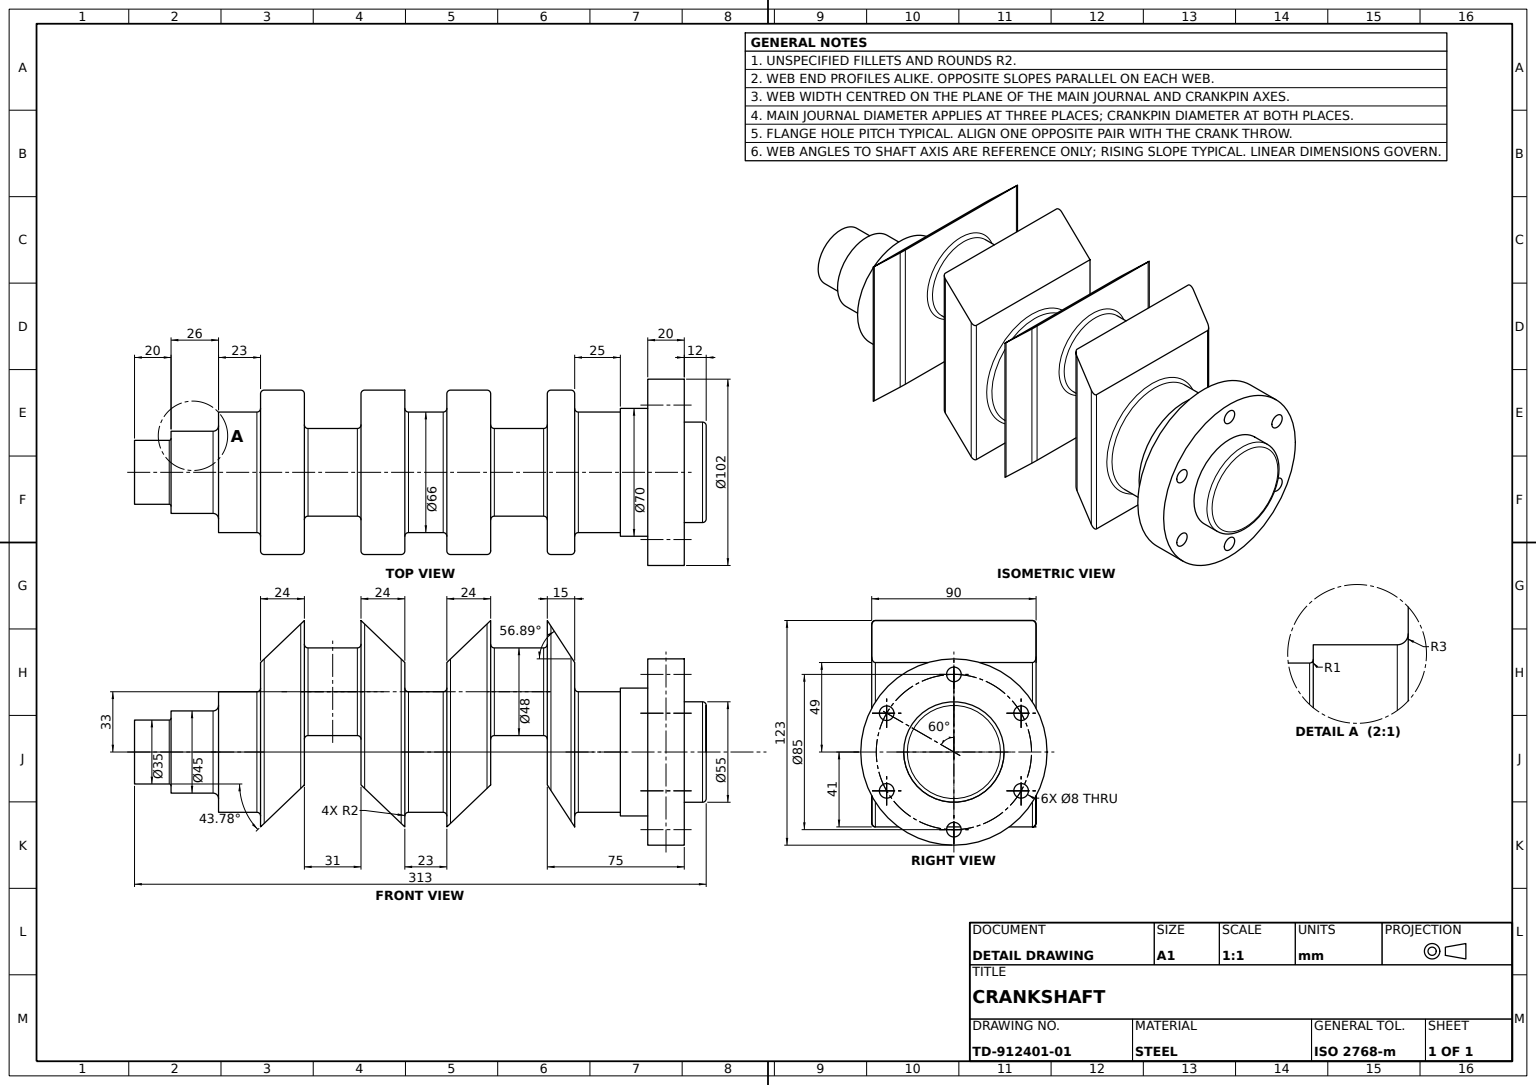
SolidWorks part; units mm, degrees
material "Plain Carbon Steel"
ref_plane "Front Plane" through (0, 0, 0) normal (0, 0, 1) x (1, 0, 0)
ref_plane "Top Plane" through (0, 0, 0) normal (0, 1, 0) x (1, 0, 0)
ref_plane "Right Plane" through (0, 0, 0) normal (1, 0, 0) x (0, 0, -1)
sketch "Front Journal Ø35 Sketch" plane through (0, 0, 0) normal (0, 0, 1) x (1, 0, 0)
  circle A0 centre (0, 0) radius 17.5
  dimension "D1" = 35
extrude "Front Journal Ø35" add sketch "Front Journal Ø35 Sketch" against normal blind 20
sketch "Shaft Step Ø45 Sketch" plane through (0, 0, -20) normal (0, 0, -1) x (-1, 0, 0)
  circle A0 centre (0, 0) radius 22.5
  dimension "D1" = 45
extrude "Shaft Step Ø45" add sketch "Shaft Step Ø45 Sketch" along normal blind 26
sketch "Front Main Journal Ø66 Sketch" plane through (0, 0, -46) normal (0, 0, -1) x (-1, 0, 0)
  circle A0 centre (0, 0) radius 33
  dimension "D1" = 66
extrude "Front Main Journal Ø66" add sketch "Front Main Journal Ø66 Sketch" along normal blind 23
sketch "Crank Web 1 Profile" plane through (0, 0, 0) normal (1, 0, 0) x (0, 0, -1)
  line L0 (69, 0) -> (69, 49)
  line L1 (69, -33) -> (69, 33) construction
  line L2 (69, 49) -> (93, 72)
  line L3 (93, 72) -> (93, -18)
  line L4 (93, -18) -> (69, -41)
  line L5 (69, -41) -> (69, 0)
  dimension "D1" = 23
  dimension "D2" = 24
  dimension "D3" = 49
  dimension "D4" = 41
  dimension "D5" = 90
extrude "Crank Web 1" add sketch "Crank Web 1 Profile" along normal mid plane 90
sketch "Crankpin 1 Ø48 Sketch" plane through (0, 0, -93) normal (0, 0, -1) x (-1, 0, 0)
  circle A0 centre (0, 33) radius 24
  circle A1 centre (0, 0) radius 33 construction
  dimension "D1" = 48
extrude "Crankpin 1 Ø48" add sketch "Crankpin 1 Ø48 Sketch" along normal blind 31
sketch "Crank Web 2 Profile" plane through (0, 0, 0) normal (1, 0, 0) x (0, 0, -1)
  line L0 (124, 72) -> (124, -18)
  line L1 (124, -18) -> (148, -41)
  line L2 (148, -41) -> (148, 49)
  line L3 (148, 49) -> (124, 72)
  dimension "D1" = 90
  dimension "D2" = 24
  dimension "D3" = 23
  dimension "D4" = 72
extrude "Crank Web 2" add sketch "Crank Web 2 Profile" along normal mid plane 90
sketch "Centre Main Journal Ø66 Sketch" plane through (0, 0, -148) normal (0, 0, -1) x (-1, 0, 0)
  circle A0 centre (0, 0) radius 33
  circle A1 centre (0, 0) radius 33 construction
  dimension "D1" = 66
extrude "Centre Main Journal Ø66" add sketch "Centre Main Journal Ø66 Sketch" along normal blind 23
sketch "Crank Web 3 Profile" plane through (0, 0, 0) normal (1, 0, 0) x (0, 0, -1)
  line L0 (171, 0) -> (171, 49)
  line L1 (171, -33) -> (171, 33) construction
  line L2 (171, 0) -> (171, -41)
  line L3 (171, 49) -> (195, 72)
  line L4 (195, 72) -> (195, -18)
  line L5 (195, -18) -> (171, -41)
  dimension "D1" = 49
  dimension "D2" = 23
  dimension "D3" = 24
  dimension "D4" = 90
extrude "Crank Web 3" add sketch "Crank Web 3 Profile" along normal mid plane 90
sketch "Crankpin 2 Sketch" plane through (0, 0, -195) normal (0, 0, -1) x (-1, 0, 0)
  circle A0 centre (0, 33) radius 24 construction
  circle A1 centre (0, 33) radius 24
extrude "Crankpin 2" add sketch "Crankpin 2 Sketch" along normal blind 31
sketch "Crank Web 4 Profile" plane through (0, 0, 0) normal (1, 0, 0) x (0, 0, -1)
  line L0 (226, 57) -> (226, 72)
  line L1 (226, 72) -> (241, 49)
  line L2 (241, 49) -> (241, -41)
  line L3 (241, -41) -> (226, -18)
  line L4 (226, -18) -> (226, 57)
  dimension "D1" = 15
  dimension "D2" = 23
  dimension "D3" = 75
  dimension "D4" = 90
extrude "Crank Web 4" add sketch "Crank Web 4 Profile" along normal mid plane 90
sketch "Rear Main Journal Sketch" plane through (0, 0, -241) normal (0, 0, -1) x (-1, 0, 0)
  circle A0 centre (0, 0) radius 33 construction
  circle A1 centre (0, 0) radius 33
extrude "Rear Main Journal" add sketch "Rear Main Journal Sketch" along normal blind 25
sketch "Flange Neck Ø70 Sketch" plane through (0, 0, -266) normal (0, 0, -1) x (-1, 0, 0)
  circle A0 centre (0, 0) radius 35
  dimension "D1" = 70
extrude "Flange Neck Ø70" add sketch "Flange Neck Ø70 Sketch" along normal blind 15
sketch "Rear Flange Ø102 Sketch" plane through (0, 0, -281) normal (0, 0, -1) x (-1, 0, 0)
  circle A0 centre (0, 0) radius 51
  dimension "D1" = 102
extrude "Rear Flange Ø102" add sketch "Rear Flange Ø102 Sketch" along normal blind 20
sketch "Flange Spigot Ø55 Sketch" plane through (0, 0, -301) normal (0, 0, -1) x (-1, 0, 0)
  circle A0 centre (0, 0) radius 27.5
  dimension "D1" = 55
extrude "Flange Spigot Ø55" add sketch "Flange Spigot Ø55 Sketch" along normal blind 12
sketch "Flange Bolt Holes Sketch" plane through (0, 0, -301) normal (0, 0, -1) x (-1, 0, 0)
  circle A0 centre (0, 0) radius 42.5 construction
  circle A1 centre (0, 42.5) radius 4
  circle A2 centre (36.8061, 21.25) radius 4
  circle A3 centre (36.8061, -21.25) radius 4
  circle A4 centre (0, -42.5) radius 4
  circle A5 centre (-36.8061, -21.25) radius 4
  circle A6 centre (-36.8061, 21.25) radius 4
  dimension "D1" = 85
  dimension "D2" = 8
  dimension "D3" = 6
extrude "Flange Bolt Holes 6xØ8 PCD85" cut sketch "Flange Bolt Holes Sketch" against normal up to next
fillet "Front Journal Fillet R1" radius 1 1 edges at (17.5, 0, -20)
fillet "Shaft Step Fillet R3" radius 3 1 edges at (-22.5, 0, -46)
fillet "Journal and Crankpin Fillets R2" radius 2 9 edges at (-33, 0, -69) (-27.5, 0, -313) (-33, 0, -241) (-24, 33, -226) (-24, 33, -195) (0, 33, -171) (0, 33, -148) (0, 57, -124) (0, 57, -93)
fillet "Crank Web 1 Edge Fillet R2" radius 2 4 edges at (-45, 4, -69) (-45, 27, -93) (45, 27, -93) (45, 4, -69)
fillet "Crank Webs 2-4 Edge Fillets R2" radius 2 11 edges at (-45, 4, -171) (-45, 27, -195) (-45, 27, -226) (-45, 4, -241) (45, 4, -241) (45, 27, -226) (45, 27, -195) (45, 4, -171) (45, 4, -148) (45, 27, -124) (-45, 27, -124)
